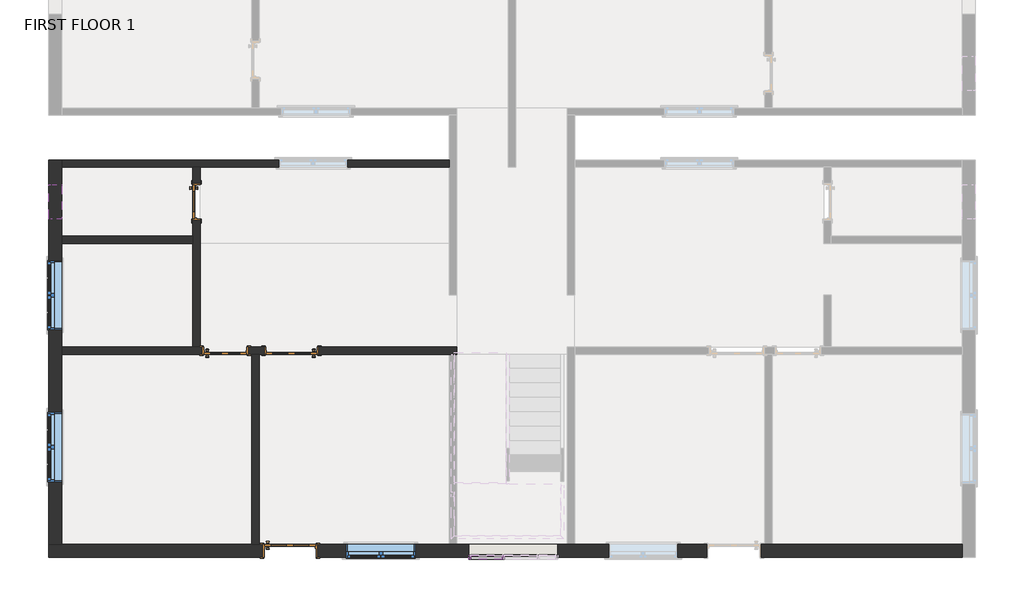
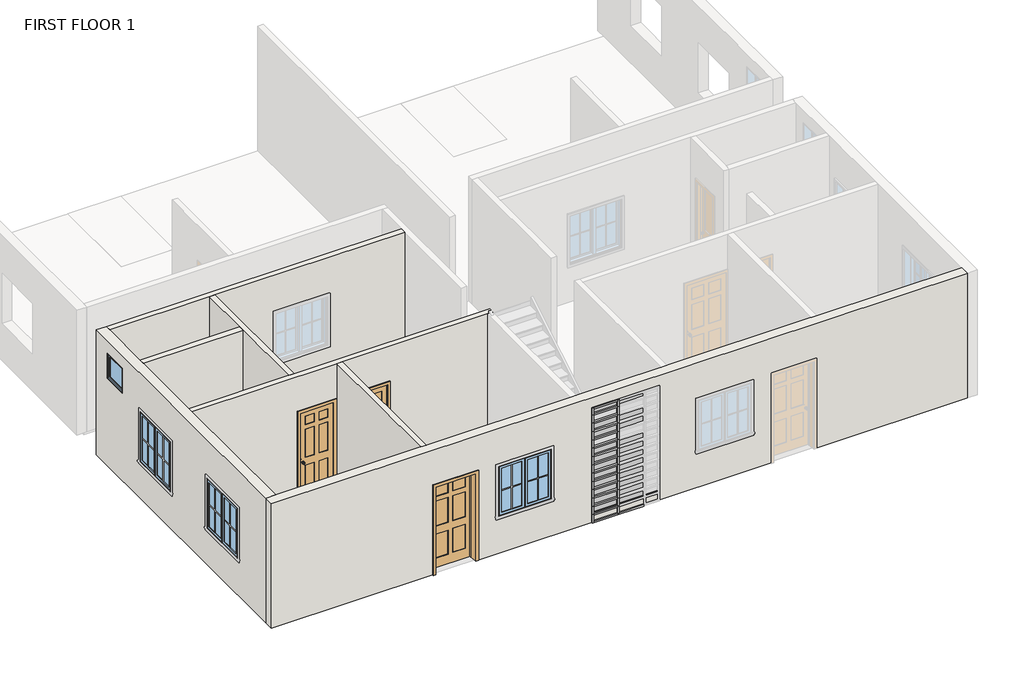
# One storey, part 1 of 4: 44 members, 24 plates, 7 walls, 4 doors, 4 windows.
"""IFC4 building model written with IfcOpenShell, lengths in millimetres."""

from ifc_helpers import new_model, si_unit, frame, origin, place, context, project, spatial, polyline, outline, extrude, faceted_brep, transform, mapped, element, save
from components import door_e337afa5, door_3b50870b, door_d86b6c54, door_03e3dfb5, member_56b223d9, member_a59c64b1, member_fa69921b, member_a67f877f, member_6a7c88b6, member_dc11c383, member_ff422208, system_panel_glazed_844a74e3, system_panel_glazed_a39216e9, system_panel_glazed_b3845325, system_panel_glazed_23b8b45c, system_panel_glazed_26c33eb0, system_panel_glazed_afc0885c, window_80340324, window_9200f5ac

model = new_model("IFC4")

# Units and contexts
model_context = context("Model", 3, world=origin())
ifc_project = project(units=[si_unit("LENGTHUNIT", "METRE", prefix="MILLI")], contexts=[model_context])

# Site, building, storey
site = spatial("IfcSite", under=ifc_project)
building = spatial("IfcBuilding", under=site)
storey = spatial("IfcBuildingStorey", under=building, Name="FIRST FLOOR 1", Elevation=3200.4)

# Doors
placement = place(None, origin())
door_shape = door_e337afa5(model_context)
element("IfcDoor", 1, ObjectType="Door-Interior-Single-2_Panel-Wood : 24\" x 84\"", at=placement, inside=storey, context=model_context, shape_type="MappedRepresentation", body=[
    mapped(door_shape, transform((-9830.0887331, -1548.6593836, 3200.4), x_axis=(0.0, -1.0, 0.0), y_axis=(1.0, 0.0, 0.0), z_axis=(0.0, 0.0, 1.0))),
])
door_2_shape = door_3b50870b(model_context)
element("IfcDoor", 2, ObjectType="Door-Interior-Single-6_Panel-Wood : 30\" x 84\"", at=placement, inside=storey, context=model_context, shape_type="MappedRepresentation", body=[
    mapped(door_2_shape, transform((-9318.9137331, -4180.7343836, 3200.4), x_axis=(1.0, 0.0, 0.0), y_axis=(0.0, 1.0, 0.0), z_axis=(0.0, 0.0, 1.0))),
])
door_3_shape = door_d86b6c54(model_context)
element("IfcDoor", 3, ObjectType="Door-Interior-Single-6_Panel-Wood : 36\" x 84\"", at=placement, inside=storey, context=model_context, shape_type="MappedRepresentation", body=[
    mapped(door_3_shape, transform((-8175.9137331, -7704.9843836, 3200.4), x_axis=(1.0, 0.0, 0.0), y_axis=(0.0, 1.0, 0.0), z_axis=(0.0, 0.0, 1.0))),
])
door_4_shape = door_03e3dfb5(model_context)
element("IfcDoor", 4, ObjectType="Door-Interior-Single-6_Panel-Wood : 36\" x 84\"", at=placement, inside=storey, context=model_context, shape_type="MappedRepresentation", body=[
    mapped(door_4_shape, transform((-8150.5137331, -4180.7343836, 3200.4), x_axis=(-1.0, 0.0, 0.0), y_axis=(0.0, -1.0, 0.0), z_axis=(0.0, 0.0, 1.0))),
])

# Members
member_shape = member_56b223d9(model_context)
element("IfcMember", 5, ObjectType="Rectangular Mullion : 1.5\" x 2.5\" rectangular", at=placement, inside=storey, context=model_context, shape_type="MappedRepresentation", body=[
    mapped(member_shape, transform((-4416.6334597, -7822.4593836, 3200.4), x_axis=(1.0, 0.0, 0.0), y_axis=(0.0, -1.0, 0.0), z_axis=(0.0, 0.0, -1.0))),
])
element("IfcMember", 6, ObjectType="Rectangular Mullion : 1.5\" x 2.5\" rectangular", at=placement, inside=storey, context=model_context, shape_type="MappedRepresentation", body=[
    mapped(member_shape, transform((-4416.6334597, -7822.4593836, 3403.6), x_axis=(1.0, 0.0, 0.0), y_axis=(0.0, -1.0, 0.0), z_axis=(0.0, 0.0, -1.0))),
])
element("IfcMember", 7, ObjectType="Rectangular Mullion : 1.5\" x 2.5\" rectangular", at=placement, inside=storey, context=model_context, shape_type="MappedRepresentation", body=[
    mapped(member_shape, transform((-4416.6334597, -7822.4593836, 3606.8), x_axis=(1.0, 0.0, 0.0), y_axis=(0.0, -1.0, 0.0), z_axis=(0.0, 0.0, -1.0))),
])
element("IfcMember", 8, ObjectType="Rectangular Mullion : 1.5\" x 2.5\" rectangular", at=placement, inside=storey, context=model_context, shape_type="MappedRepresentation", body=[
    mapped(member_shape, transform((-4416.6334597, -7822.4593836, 3810.0), x_axis=(1.0, 0.0, 0.0), y_axis=(0.0, -1.0, 0.0), z_axis=(0.0, 0.0, -1.0))),
])
element("IfcMember", 9, ObjectType="Rectangular Mullion : 1.5\" x 2.5\" rectangular", at=placement, inside=storey, context=model_context, shape_type="MappedRepresentation", body=[
    mapped(member_shape, transform((-4416.6334597, -7822.4593836, 4013.2), x_axis=(1.0, 0.0, 0.0), y_axis=(0.0, -1.0, 0.0), z_axis=(0.0, 0.0, -1.0))),
])
element("IfcMember", 10, ObjectType="Rectangular Mullion : 1.5\" x 2.5\" rectangular", at=placement, inside=storey, context=model_context, shape_type="MappedRepresentation", body=[
    mapped(member_shape, transform((-4416.6334597, -7822.4593836, 4216.4), x_axis=(1.0, 0.0, 0.0), y_axis=(0.0, -1.0, 0.0), z_axis=(0.0, 0.0, -1.0))),
])
element("IfcMember", 11, ObjectType="Rectangular Mullion : 1.5\" x 2.5\" rectangular", at=placement, inside=storey, context=model_context, shape_type="MappedRepresentation", body=[
    mapped(member_shape, transform((-4416.6334597, -7822.4593836, 4419.6), x_axis=(1.0, 0.0, 0.0), y_axis=(0.0, -1.0, 0.0), z_axis=(0.0, 0.0, -1.0))),
])
element("IfcMember", 12, ObjectType="Rectangular Mullion : 1.5\" x 2.5\" rectangular", at=placement, inside=storey, context=model_context, shape_type="MappedRepresentation", body=[
    mapped(member_shape, transform((-4416.6334597, -7822.4593836, 4622.8), x_axis=(1.0, 0.0, 0.0), y_axis=(0.0, -1.0, 0.0), z_axis=(0.0, 0.0, -1.0))),
])
element("IfcMember", 13, ObjectType="Rectangular Mullion : 1.5\" x 2.5\" rectangular", at=placement, inside=storey, context=model_context, shape_type="MappedRepresentation", body=[
    mapped(member_shape, transform((-4416.6334597, -7822.4593836, 4826.0), x_axis=(1.0, 0.0, 0.0), y_axis=(0.0, -1.0, 0.0), z_axis=(0.0, 0.0, -1.0))),
])
element("IfcMember", 14, ObjectType="Rectangular Mullion : 1.5\" x 2.5\" rectangular", at=placement, inside=storey, context=model_context, shape_type="MappedRepresentation", body=[
    mapped(member_shape, transform((-4416.6334597, -7822.4593836, 5029.2), x_axis=(1.0, 0.0, 0.0), y_axis=(0.0, -1.0, 0.0), z_axis=(0.0, 0.0, -1.0))),
])
element("IfcMember", 15, ObjectType="Rectangular Mullion : 1.5\" x 2.5\" rectangular", at=placement, inside=storey, context=model_context, shape_type="MappedRepresentation", body=[
    mapped(member_shape, transform((-4416.6334597, -7822.4593836, 5232.4), x_axis=(1.0, 0.0, 0.0), y_axis=(0.0, -1.0, 0.0), z_axis=(0.0, 0.0, -1.0))),
])
element("IfcMember", 16, ObjectType="Rectangular Mullion : 1.5\" x 2.5\" rectangular", at=placement, inside=storey, context=model_context, shape_type="MappedRepresentation", body=[
    mapped(member_shape, transform((-4416.6334597, -7822.4593836, 5435.6), x_axis=(1.0, 0.0, 0.0), y_axis=(0.0, -1.0, 0.0), z_axis=(0.0, 0.0, -1.0))),
])
element("IfcMember", 17, ObjectType="Rectangular Mullion : 1.5\" x 2.5\" rectangular", at=placement, inside=storey, context=model_context, shape_type="MappedRepresentation", body=[
    mapped(member_shape, transform((-4416.6334597, -7822.4593836, 5638.8), x_axis=(1.0, 0.0, 0.0), y_axis=(0.0, -1.0, 0.0), z_axis=(0.0, 0.0, -1.0))),
])
member_2_shape = member_a59c64b1(model_context)
element("IfcMember", 18, ObjectType="Rectangular Mullion : 1.5\" x 2.5\" rectangular", at=placement, inside=storey, context=model_context, shape_type="MappedRepresentation", body=[
    mapped(member_2_shape, transform((-4416.6334597, -7822.4593836, 5842.0), x_axis=(1.0, 0.0, 0.0), y_axis=(0.0, -1.0, 0.0), z_axis=(0.0, 0.0, -1.0))),
])
member_3_shape = member_fa69921b(model_context)
element("IfcMember", 19, ObjectType="Rectangular Mullion : 1.5\" x 2.5\" rectangular", at=placement, inside=storey, context=model_context, shape_type="MappedRepresentation", body=[
    mapped(member_3_shape, transform((-4435.6834597, -7822.4593836, 6007.7826151), x_axis=(0.0, 0.0, 1.0), y_axis=(0.0, -1.0, 0.0), z_axis=(1.0, 0.0, 0.0))),
])
element("IfcMember", 20, ObjectType="Rectangular Mullion : 1.5\" x 2.5\" rectangular", at=placement, inside=storey, context=model_context, shape_type="MappedRepresentation", body=[
    mapped(member_3_shape, transform((-4988.13346, -7822.4593836, 3200.4), x_axis=(0.0, 0.0, -1.0), y_axis=(0.0, -1.0, 0.0), z_axis=(-1.0, 0.0, 0.0))),
])
member_4_shape = member_a67f877f(model_context)
element("IfcMember", 21, ObjectType="Rectangular Mullion : 1.5\" x 2.5\" rectangular", at=placement, inside=storey, context=model_context, shape_type="MappedRepresentation", body=[
    mapped(member_4_shape, transform((-4397.5834597, -7822.4593836, 3200.4), x_axis=(0.0, 0.0, -1.0), y_axis=(0.0, -1.0, 0.0), z_axis=(-1.0, 0.0, 0.0))),
])
member_5_shape = member_6a7c88b6(model_context)
element("IfcMember", 22, ObjectType="Rectangular Mullion : 1.5\" x 2.5\" rectangular", at=placement, inside=storey, context=model_context, shape_type="MappedRepresentation", body=[
    mapped(member_5_shape, transform((-4435.6834597, -7822.4593836, 3403.6), x_axis=(0.0, 0.0, 1.0), y_axis=(0.0, -1.0, 0.0), z_axis=(1.0, 0.0, 0.0))),
])
element("IfcMember", 23, ObjectType="Rectangular Mullion : 1.5\" x 2.5\" rectangular", at=placement, inside=storey, context=model_context, shape_type="MappedRepresentation", body=[
    mapped(member_5_shape, transform((-4435.6834597, -7822.4593836, 3606.8), x_axis=(0.0, 0.0, 1.0), y_axis=(0.0, -1.0, 0.0), z_axis=(1.0, 0.0, 0.0))),
])
element("IfcMember", 24, ObjectType="Rectangular Mullion : 1.5\" x 2.5\" rectangular", at=placement, inside=storey, context=model_context, shape_type="MappedRepresentation", body=[
    mapped(member_5_shape, transform((-4435.6834597, -7822.4593836, 3810.0), x_axis=(0.0, 0.0, 1.0), y_axis=(0.0, -1.0, 0.0), z_axis=(1.0, 0.0, 0.0))),
])
element("IfcMember", 25, ObjectType="Rectangular Mullion : 1.5\" x 2.5\" rectangular", at=placement, inside=storey, context=model_context, shape_type="MappedRepresentation", body=[
    mapped(member_5_shape, transform((-4435.6834597, -7822.4593836, 4013.2), x_axis=(0.0, 0.0, 1.0), y_axis=(0.0, -1.0, 0.0), z_axis=(1.0, 0.0, 0.0))),
])
element("IfcMember", 26, ObjectType="Rectangular Mullion : 1.5\" x 2.5\" rectangular", at=placement, inside=storey, context=model_context, shape_type="MappedRepresentation", body=[
    mapped(member_5_shape, transform((-4435.6834597, -7822.4593836, 4216.4), x_axis=(0.0, 0.0, 1.0), y_axis=(0.0, -1.0, 0.0), z_axis=(1.0, 0.0, 0.0))),
])
element("IfcMember", 27, ObjectType="Rectangular Mullion : 1.5\" x 2.5\" rectangular", at=placement, inside=storey, context=model_context, shape_type="MappedRepresentation", body=[
    mapped(member_5_shape, transform((-4435.6834597, -7822.4593836, 4419.6), x_axis=(0.0, 0.0, 1.0), y_axis=(0.0, -1.0, 0.0), z_axis=(1.0, 0.0, 0.0))),
])
element("IfcMember", 28, ObjectType="Rectangular Mullion : 1.5\" x 2.5\" rectangular", at=placement, inside=storey, context=model_context, shape_type="MappedRepresentation", body=[
    mapped(member_5_shape, transform((-4435.6834597, -7822.4593836, 4622.8), x_axis=(0.0, 0.0, 1.0), y_axis=(0.0, -1.0, 0.0), z_axis=(1.0, 0.0, 0.0))),
])
element("IfcMember", 29, ObjectType="Rectangular Mullion : 1.5\" x 2.5\" rectangular", at=placement, inside=storey, context=model_context, shape_type="MappedRepresentation", body=[
    mapped(member_5_shape, transform((-4435.6834597, -7822.4593836, 4826.0), x_axis=(0.0, 0.0, 1.0), y_axis=(0.0, -1.0, 0.0), z_axis=(1.0, 0.0, 0.0))),
])
element("IfcMember", 30, ObjectType="Rectangular Mullion : 1.5\" x 2.5\" rectangular", at=placement, inside=storey, context=model_context, shape_type="MappedRepresentation", body=[
    mapped(member_5_shape, transform((-4435.6834597, -7822.4593836, 5029.2), x_axis=(0.0, 0.0, 1.0), y_axis=(0.0, -1.0, 0.0), z_axis=(1.0, 0.0, 0.0))),
])
element("IfcMember", 31, ObjectType="Rectangular Mullion : 1.5\" x 2.5\" rectangular", at=placement, inside=storey, context=model_context, shape_type="MappedRepresentation", body=[
    mapped(member_5_shape, transform((-4435.6834597, -7822.4593836, 5232.4), x_axis=(0.0, 0.0, 1.0), y_axis=(0.0, -1.0, 0.0), z_axis=(1.0, 0.0, 0.0))),
])
element("IfcMember", 32, ObjectType="Rectangular Mullion : 1.5\" x 2.5\" rectangular", at=placement, inside=storey, context=model_context, shape_type="MappedRepresentation", body=[
    mapped(member_5_shape, transform((-4435.6834597, -7822.4593836, 5435.6), x_axis=(0.0, 0.0, 1.0), y_axis=(0.0, -1.0, 0.0), z_axis=(1.0, 0.0, 0.0))),
])
element("IfcMember", 33, ObjectType="Rectangular Mullion : 1.5\" x 2.5\" rectangular", at=placement, inside=storey, context=model_context, shape_type="MappedRepresentation", body=[
    mapped(member_5_shape, transform((-4435.6834597, -7822.4593836, 5638.8), x_axis=(0.0, 0.0, 1.0), y_axis=(0.0, -1.0, 0.0), z_axis=(1.0, 0.0, 0.0))),
])
element("IfcMember", 34, ObjectType="Rectangular Mullion : 1.5\" x 2.5\" rectangular", at=placement, inside=storey, context=model_context, shape_type="MappedRepresentation", body=[
    mapped(member_5_shape, transform((-4435.6834597, -7822.4593836, 5842.0), x_axis=(0.0, 0.0, 1.0), y_axis=(0.0, -1.0, 0.0), z_axis=(1.0, 0.0, 0.0))),
])
member_6_shape = member_dc11c383(model_context)
element("IfcMember", 35, ObjectType="Rectangular Mullion : 1.5\" x 2.5\" rectangular", at=placement, inside=storey, context=model_context, shape_type="MappedRepresentation", body=[
    mapped(member_6_shape, transform((-5026.23346, -7822.4593836, 6007.7826151), x_axis=(-1.0, 0.0, 0.0), y_axis=(0.0, -1.0, 0.0), z_axis=(0.0, 0.0, 1.0))),
])
member_7_shape = member_ff422208(model_context)
element("IfcMember", 36, ObjectType="Rectangular Mullion : 1.5\" x 2.5\" rectangular", at=placement, inside=storey, context=model_context, shape_type="MappedRepresentation", body=[
    mapped(member_7_shape, transform((-5026.23346, -7822.4593836, 3403.6), x_axis=(-1.0, 0.0, 0.0), y_axis=(0.0, -1.0, 0.0), z_axis=(0.0, 0.0, 1.0))),
])
element("IfcMember", 37, ObjectType="Rectangular Mullion : 1.5\" x 2.5\" rectangular", at=placement, inside=storey, context=model_context, shape_type="MappedRepresentation", body=[
    mapped(member_7_shape, transform((-5026.23346, -7822.4593836, 3606.8), x_axis=(-1.0, 0.0, 0.0), y_axis=(0.0, -1.0, 0.0), z_axis=(0.0, 0.0, 1.0))),
])
element("IfcMember", 38, ObjectType="Rectangular Mullion : 1.5\" x 2.5\" rectangular", at=placement, inside=storey, context=model_context, shape_type="MappedRepresentation", body=[
    mapped(member_7_shape, transform((-5026.23346, -7822.4593836, 3810.0), x_axis=(-1.0, 0.0, 0.0), y_axis=(0.0, -1.0, 0.0), z_axis=(0.0, 0.0, 1.0))),
])
element("IfcMember", 39, ObjectType="Rectangular Mullion : 1.5\" x 2.5\" rectangular", at=placement, inside=storey, context=model_context, shape_type="MappedRepresentation", body=[
    mapped(member_7_shape, transform((-5026.23346, -7822.4593836, 4013.2), x_axis=(-1.0, 0.0, 0.0), y_axis=(0.0, -1.0, 0.0), z_axis=(0.0, 0.0, 1.0))),
])
element("IfcMember", 40, ObjectType="Rectangular Mullion : 1.5\" x 2.5\" rectangular", at=placement, inside=storey, context=model_context, shape_type="MappedRepresentation", body=[
    mapped(member_7_shape, transform((-5026.23346, -7822.4593836, 4216.4), x_axis=(-1.0, 0.0, 0.0), y_axis=(0.0, -1.0, 0.0), z_axis=(0.0, 0.0, 1.0))),
])
element("IfcMember", 41, ObjectType="Rectangular Mullion : 1.5\" x 2.5\" rectangular", at=placement, inside=storey, context=model_context, shape_type="MappedRepresentation", body=[
    mapped(member_7_shape, transform((-5026.23346, -7822.4593836, 4419.6), x_axis=(-1.0, 0.0, 0.0), y_axis=(0.0, -1.0, 0.0), z_axis=(0.0, 0.0, 1.0))),
])
element("IfcMember", 42, ObjectType="Rectangular Mullion : 1.5\" x 2.5\" rectangular", at=placement, inside=storey, context=model_context, shape_type="MappedRepresentation", body=[
    mapped(member_7_shape, transform((-5026.23346, -7822.4593836, 4622.8), x_axis=(-1.0, 0.0, 0.0), y_axis=(0.0, -1.0, 0.0), z_axis=(0.0, 0.0, 1.0))),
])
element("IfcMember", 43, ObjectType="Rectangular Mullion : 1.5\" x 2.5\" rectangular", at=placement, inside=storey, context=model_context, shape_type="MappedRepresentation", body=[
    mapped(member_7_shape, transform((-5026.23346, -7822.4593836, 4826.0), x_axis=(-1.0, 0.0, 0.0), y_axis=(0.0, -1.0, 0.0), z_axis=(0.0, 0.0, 1.0))),
])
element("IfcMember", 44, ObjectType="Rectangular Mullion : 1.5\" x 2.5\" rectangular", at=placement, inside=storey, context=model_context, shape_type="MappedRepresentation", body=[
    mapped(member_7_shape, transform((-5026.23346, -7822.4593836, 5029.2), x_axis=(-1.0, 0.0, 0.0), y_axis=(0.0, -1.0, 0.0), z_axis=(0.0, 0.0, 1.0))),
])
element("IfcMember", 45, ObjectType="Rectangular Mullion : 1.5\" x 2.5\" rectangular", at=placement, inside=storey, context=model_context, shape_type="MappedRepresentation", body=[
    mapped(member_7_shape, transform((-5026.23346, -7822.4593836, 5232.4), x_axis=(-1.0, 0.0, 0.0), y_axis=(0.0, -1.0, 0.0), z_axis=(0.0, 0.0, 1.0))),
])
element("IfcMember", 46, ObjectType="Rectangular Mullion : 1.5\" x 2.5\" rectangular", at=placement, inside=storey, context=model_context, shape_type="MappedRepresentation", body=[
    mapped(member_7_shape, transform((-5026.23346, -7822.4593836, 5435.6), x_axis=(-1.0, 0.0, 0.0), y_axis=(0.0, -1.0, 0.0), z_axis=(0.0, 0.0, 1.0))),
])
element("IfcMember", 47, ObjectType="Rectangular Mullion : 1.5\" x 2.5\" rectangular", at=placement, inside=storey, context=model_context, shape_type="MappedRepresentation", body=[
    mapped(member_7_shape, transform((-5026.23346, -7822.4593836, 5638.8), x_axis=(-1.0, 0.0, 0.0), y_axis=(0.0, -1.0, 0.0), z_axis=(0.0, 0.0, 1.0))),
])
element("IfcMember", 48, ObjectType="Rectangular Mullion : 1.5\" x 2.5\" rectangular", at=placement, inside=storey, context=model_context, shape_type="MappedRepresentation", body=[
    mapped(member_7_shape, transform((-5026.23346, -7822.4593836, 5842.0), x_axis=(-1.0, 0.0, 0.0), y_axis=(0.0, -1.0, 0.0), z_axis=(0.0, 0.0, 1.0))),
])

# Plates
system_panel_glazed_shape = system_panel_glazed_844a74e3(model_context)
element("IfcPlate", 49, ObjectType="System Panel : Glazed", at=placement, inside=storey, context=model_context, shape_type="MappedRepresentation", body=[
    mapped(system_panel_glazed_shape, transform((-4711.9084599, -7822.4593836, 3238.5), x_axis=(1.0, 0.0, 0.0), y_axis=(0.0, 1.0, 0.0), z_axis=(0.0, 0.0, 1.0))),
])
system_panel_glazed_2_shape = system_panel_glazed_a39216e9(model_context)
element("IfcPlate", 50, ObjectType="System Panel : Glazed", at=placement, inside=storey, context=model_context, shape_type="MappedRepresentation", body=[
    mapped(system_panel_glazed_2_shape, transform((-4111.8334597, -7822.4593836, 3238.5), x_axis=(1.0, 0.0, 0.0), y_axis=(0.0, 1.0, 0.0), z_axis=(0.0, 0.0, 1.0))),
])
system_panel_glazed_3_shape = system_panel_glazed_b3845325(model_context)
element("IfcPlate", 51, ObjectType="System Panel : Glazed", at=placement, inside=storey, context=model_context, shape_type="MappedRepresentation", body=[
    mapped(system_panel_glazed_3_shape, transform((-4711.9084599, -7822.4593836, 3422.65), x_axis=(1.0, 0.0, 0.0), y_axis=(0.0, 1.0, 0.0), z_axis=(0.0, 0.0, 1.0))),
])
element("IfcPlate", 52, ObjectType="System Panel : Glazed", at=placement, inside=storey, context=model_context, shape_type="MappedRepresentation", body=[
    mapped(system_panel_glazed_3_shape, transform((-4711.9084599, -7822.4593836, 3625.85), x_axis=(1.0, 0.0, 0.0), y_axis=(0.0, 1.0, 0.0), z_axis=(0.0, 0.0, 1.0))),
])
element("IfcPlate", 53, ObjectType="System Panel : Glazed", at=placement, inside=storey, context=model_context, shape_type="MappedRepresentation", body=[
    mapped(system_panel_glazed_3_shape, transform((-4711.9084599, -7822.4593836, 4032.25), x_axis=(1.0, 0.0, 0.0), y_axis=(0.0, 1.0, 0.0), z_axis=(0.0, 0.0, 1.0))),
])
element("IfcPlate", 54, ObjectType="System Panel : Glazed", at=placement, inside=storey, context=model_context, shape_type="MappedRepresentation", body=[
    mapped(system_panel_glazed_3_shape, transform((-4711.9084599, -7822.4593836, 4235.45), x_axis=(1.0, 0.0, 0.0), y_axis=(0.0, 1.0, 0.0), z_axis=(0.0, 0.0, 1.0))),
])
element("IfcPlate", 55, ObjectType="System Panel : Glazed", at=placement, inside=storey, context=model_context, shape_type="MappedRepresentation", body=[
    mapped(system_panel_glazed_3_shape, transform((-4711.9084599, -7822.4593836, 4641.85), x_axis=(1.0, 0.0, 0.0), y_axis=(0.0, 1.0, 0.0), z_axis=(0.0, 0.0, 1.0))),
])
element("IfcPlate", 56, ObjectType="System Panel : Glazed", at=placement, inside=storey, context=model_context, shape_type="MappedRepresentation", body=[
    mapped(system_panel_glazed_3_shape, transform((-4711.9084599, -7822.4593836, 4845.05), x_axis=(1.0, 0.0, 0.0), y_axis=(0.0, 1.0, 0.0), z_axis=(0.0, 0.0, 1.0))),
])
element("IfcPlate", 57, ObjectType="System Panel : Glazed", at=placement, inside=storey, context=model_context, shape_type="MappedRepresentation", body=[
    mapped(system_panel_glazed_3_shape, transform((-4711.9084599, -7822.4593836, 5251.45), x_axis=(1.0, 0.0, 0.0), y_axis=(0.0, 1.0, 0.0), z_axis=(0.0, 0.0, 1.0))),
])
element("IfcPlate", 58, ObjectType="System Panel : Glazed", at=placement, inside=storey, context=model_context, shape_type="MappedRepresentation", body=[
    mapped(system_panel_glazed_3_shape, transform((-4711.9084599, -7822.4593836, 5454.65), x_axis=(1.0, 0.0, 0.0), y_axis=(0.0, 1.0, 0.0), z_axis=(0.0, 0.0, 1.0))),
])
element("IfcPlate", 59, ObjectType="System Panel : Glazed", at=placement, inside=storey, context=model_context, shape_type="MappedRepresentation", body=[
    mapped(system_panel_glazed_3_shape, transform((-4711.9084599, -7822.4593836, 3829.05), x_axis=(1.0, 0.0, 0.0), y_axis=(0.0, 1.0, 0.0), z_axis=(0.0, 0.0, 1.0))),
])
element("IfcPlate", 60, ObjectType="System Panel : Glazed", at=placement, inside=storey, context=model_context, shape_type="MappedRepresentation", body=[
    mapped(system_panel_glazed_3_shape, transform((-4711.9084599, -7822.4593836, 4438.65), x_axis=(1.0, 0.0, 0.0), y_axis=(0.0, 1.0, 0.0), z_axis=(0.0, 0.0, 1.0))),
])
system_panel_glazed_4_shape = system_panel_glazed_23b8b45c(model_context)
element("IfcPlate", 61, ObjectType="System Panel : Glazed", at=placement, inside=storey, context=model_context, shape_type="MappedRepresentation", body=[
    mapped(system_panel_glazed_4_shape, transform((-4111.8334597, -7822.4593836, 3422.65), x_axis=(1.0, 0.0, 0.0), y_axis=(0.0, 1.0, 0.0), z_axis=(0.0, 0.0, 1.0))),
])
element("IfcPlate", 62, ObjectType="System Panel : Glazed", at=placement, inside=storey, context=model_context, shape_type="MappedRepresentation", body=[
    mapped(system_panel_glazed_4_shape, transform((-4111.8334597, -7822.4593836, 3625.85), x_axis=(1.0, 0.0, 0.0), y_axis=(0.0, 1.0, 0.0), z_axis=(0.0, 0.0, 1.0))),
])
element("IfcPlate", 63, ObjectType="System Panel : Glazed", at=placement, inside=storey, context=model_context, shape_type="MappedRepresentation", body=[
    mapped(system_panel_glazed_4_shape, transform((-4111.8334597, -7822.4593836, 4032.25), x_axis=(1.0, 0.0, 0.0), y_axis=(0.0, 1.0, 0.0), z_axis=(0.0, 0.0, 1.0))),
])
element("IfcPlate", 64, ObjectType="System Panel : Glazed", at=placement, inside=storey, context=model_context, shape_type="MappedRepresentation", body=[
    mapped(system_panel_glazed_4_shape, transform((-4111.8334597, -7822.4593836, 4235.45), x_axis=(1.0, 0.0, 0.0), y_axis=(0.0, 1.0, 0.0), z_axis=(0.0, 0.0, 1.0))),
])
element("IfcPlate", 65, ObjectType="System Panel : Glazed", at=placement, inside=storey, context=model_context, shape_type="MappedRepresentation", body=[
    mapped(system_panel_glazed_4_shape, transform((-4111.8334597, -7822.4593836, 4641.85), x_axis=(1.0, 0.0, 0.0), y_axis=(0.0, 1.0, 0.0), z_axis=(0.0, 0.0, 1.0))),
])
element("IfcPlate", 66, ObjectType="System Panel : Glazed", at=placement, inside=storey, context=model_context, shape_type="MappedRepresentation", body=[
    mapped(system_panel_glazed_4_shape, transform((-4111.8334597, -7822.4593836, 4845.05), x_axis=(1.0, 0.0, 0.0), y_axis=(0.0, 1.0, 0.0), z_axis=(0.0, 0.0, 1.0))),
])
element("IfcPlate", 67, ObjectType="System Panel : Glazed", at=placement, inside=storey, context=model_context, shape_type="MappedRepresentation", body=[
    mapped(system_panel_glazed_4_shape, transform((-4111.8334597, -7822.4593836, 5251.45), x_axis=(1.0, 0.0, 0.0), y_axis=(0.0, 1.0, 0.0), z_axis=(0.0, 0.0, 1.0))),
])
element("IfcPlate", 68, ObjectType="System Panel : Glazed", at=placement, inside=storey, context=model_context, shape_type="MappedRepresentation", body=[
    mapped(system_panel_glazed_4_shape, transform((-4111.8334597, -7822.4593836, 5454.65), x_axis=(1.0, 0.0, 0.0), y_axis=(0.0, 1.0, 0.0), z_axis=(0.0, 0.0, 1.0))),
])
element("IfcPlate", 69, ObjectType="System Panel : Glazed", at=placement, inside=storey, context=model_context, shape_type="MappedRepresentation", body=[
    mapped(system_panel_glazed_4_shape, transform((-4111.8334597, -7822.4593836, 3829.05), x_axis=(1.0, 0.0, 0.0), y_axis=(0.0, 1.0, 0.0), z_axis=(0.0, 0.0, 1.0))),
])
element("IfcPlate", 70, ObjectType="System Panel : Glazed", at=placement, inside=storey, context=model_context, shape_type="MappedRepresentation", body=[
    mapped(system_panel_glazed_4_shape, transform((-4111.8334597, -7822.4593836, 4438.65), x_axis=(1.0, 0.0, 0.0), y_axis=(0.0, 1.0, 0.0), z_axis=(0.0, 0.0, 1.0))),
])
system_panel_glazed_5_shape = system_panel_glazed_26c33eb0(model_context)
element("IfcPlate", 71, ObjectType="System Panel : Glazed", at=placement, inside=storey, context=model_context, shape_type="MappedRepresentation", body=[
    mapped(system_panel_glazed_5_shape, transform((-4711.9084599, -7822.4593836, 5861.05), x_axis=(1.0, 0.0, 0.0), y_axis=(0.0, 1.0, 0.0), z_axis=(0.0, 0.0, 1.0))),
])
system_panel_glazed_6_shape = system_panel_glazed_afc0885c(model_context)
element("IfcPlate", 72, ObjectType="System Panel : Glazed", at=placement, inside=storey, context=model_context, shape_type="MappedRepresentation", body=[
    mapped(system_panel_glazed_6_shape, transform((-4111.8334597, -7822.4593836, 5861.05), x_axis=(1.0, 0.0, 0.0), y_axis=(0.0, 1.0, 0.0), z_axis=(0.0, 0.0, 1.0))),
])

# Walls
element("IfcWall", 73, ObjectType="Inner Wall 5\"", at=placement, inside=storey, context=model_context, shape_type="Brep", body=[
    faceted_brep([(-12201.8137331, -939.0593836, 3200.4), (-9890.4137331, -939.0593836, 3200.4), (-9763.4137331, -939.0593836, 3200.4), (-5369.2137331, -939.0593836, 3200.4), (-5369.2137331, -939.0593836, 6248.4), (-9763.4137331, -939.0593836, 6248.4), (-9890.4137331, -939.0593836, 6248.4), (-12201.8137331, -939.0593836, 6248.4), (-7159.9137331, -939.0593836, 5334.0), (-7159.9137331, -939.0593836, 4114.8), (-8379.1137331, -939.0593836, 4114.8), (-8379.1137331, -939.0593836, 5334.0), (-12201.8137331, -812.0593836, 3200.4), (-12201.8137331, -812.0593836, 6248.4), (-5369.2137331, -812.0593836, 6248.4), (-5369.2137331, -812.0593836, 3200.4), (-7159.9137331, -812.0593836, 5334.0), (-8379.1137331, -812.0593836, 5334.0), (-8379.1137331, -812.0593836, 4114.8), (-7159.9137331, -812.0593836, 4114.8)], [[[0, 1, 2, 3, 4, 5, 6, 7], [8, 9, 10, 11]], [[12, 13, 14, 15], [16, 17, 18, 19]], [[3, 2, 1, 0, 12, 15]], [[7, 6, 5, 4, 14, 13]], [[0, 7, 13, 12]], [[4, 3, 15, 14]], [[9, 8, 16, 19]], [[10, 9, 19, 18]], [[11, 10, 18, 17]], [[8, 11, 17, 16]]]),
])
element("IfcWall", 74, ObjectType="Inner Wall 5\"", at=placement, inside=storey, context=model_context, shape_type="SweptSolid", body=[
    extrude(outline(polyline([(-8722.0137331, -4241.0593836), (-8722.0137331, -7593.8593836), (-8849.0137331, -7593.8593836), (-8849.0137331, -4241.0593836), (-8722.0137331, -4241.0593836)])), frame((0.0, 0.0, 3200.4), z_axis=(0.0, 0.0, 1.0), x_axis=(1.0, 0.0, 0.0)), (0.0, 0.0, 1.0), 3048.0),
])
element("IfcWall", 75, ObjectType="Inner Wall 5\"", at=placement, inside=storey, context=model_context, shape_type="Brep", body=[
    faceted_brep([(-12201.8137331, -4114.0593836, 6248.4), (-9890.4137331, -4114.0593836, 6248.4), (-9763.4137331, -4114.0593836, 6248.4), (-5242.2137331, -4114.0593836, 6248.4), (-5242.2137331, -4114.0593836, 3200.4), (-7667.9137331, -4114.0593836, 3200.4), (-7667.9137331, -4114.0593836, 5359.4), (-8633.1137331, -4114.0593836, 5359.4), (-8633.1137331, -4114.0593836, 3200.4), (-8912.5137331, -4114.0593836, 3200.4), (-8912.5137331, -4114.0593836, 5359.4), (-9725.3137331, -4114.0593836, 5359.4), (-9725.3137331, -4114.0593836, 3200.4), (-9763.4137331, -4114.0593836, 3200.4), (-9890.4137331, -4114.0593836, 3200.4), (-12201.8137331, -4114.0593836, 3200.4), (-5242.2137331, -4241.0593836, 6248.4), (-5369.2137331, -4241.0593836, 6248.4), (-8722.0137331, -4241.0593836, 6248.4), (-8849.0137331, -4241.0593836, 6248.4), (-12201.8137331, -4241.0593836, 6248.4), (-12201.8137331, -4241.0593836, 3200.4), (-9725.3137331, -4241.0593836, 3200.4), (-9725.3137331, -4241.0593836, 5359.4), (-8912.5137331, -4241.0593836, 5359.4), (-8912.5137331, -4241.0593836, 3200.4), (-8849.0137331, -4241.0593836, 3200.4), (-8722.0137331, -4241.0593836, 3200.4), (-8633.1137331, -4241.0593836, 3200.4), (-8633.1137331, -4241.0593836, 5359.4), (-7667.9137331, -4241.0593836, 5359.4), (-7667.9137331, -4241.0593836, 3200.4), (-5369.2137331, -4241.0593836, 3200.4), (-5242.2137331, -4241.0593836, 3200.4)], [[[0, 1, 2, 3, 4, 5, 6, 7, 8, 9, 10, 11, 12, 13, 14, 15]], [[16, 17, 18, 19, 20, 21, 22, 23, 24, 25, 26, 27, 28, 29, 30, 31, 32, 33]], [[21, 15, 14, 13, 12, 22]], [[4, 33, 32, 31, 5]], [[25, 9, 8, 28, 27, 26]], [[3, 2, 1, 0, 20, 19, 18, 17, 16]], [[0, 15, 21, 20]], [[4, 3, 16, 33]], [[10, 9, 25, 24]], [[11, 10, 24, 23]], [[12, 11, 23, 22]], [[7, 29, 28, 8]], [[29, 7, 6, 30]], [[30, 6, 5, 31]]]),
])
element("IfcWall", 76, ObjectType="Inner Wall 5\"", at=placement, inside=storey, context=model_context, shape_type="Brep", body=[
    faceted_brep([(-9763.4137331, -939.0593836, 6248.4), (-9763.4137331, -4114.0593836, 6248.4), (-9763.4137331, -4114.0593836, 3200.4), (-9763.4137331, -1878.8593836, 3200.4), (-9763.4137331, -1878.8593836, 5359.4), (-9763.4137331, -1218.4593836, 5359.4), (-9763.4137331, -1218.4593836, 3200.4), (-9763.4137331, -939.0593836, 3200.4), (-9890.4137331, -4114.0593836, 6248.4), (-9890.4137331, -2285.2593836, 6248.4), (-9890.4137331, -2158.2593836, 6248.4), (-9890.4137331, -939.0593836, 6248.4), (-9890.4137331, -939.0593836, 3200.4), (-9890.4137331, -1218.4593836, 3200.4), (-9890.4137331, -1218.4593836, 5359.4), (-9890.4137331, -1878.8593836, 5359.4), (-9890.4137331, -1878.8593836, 3200.4), (-9890.4137331, -2158.2593836, 3200.4), (-9890.4137331, -2285.2593836, 3200.4), (-9890.4137331, -4114.0593836, 3200.4)], [[[0, 1, 2, 3, 4, 5, 6, 7]], [[8, 9, 10, 11, 12, 13, 14, 15, 16, 17, 18, 19]], [[2, 19, 18, 17, 16, 3]], [[12, 7, 6, 13]], [[1, 0, 11, 10, 9, 8]], [[2, 1, 8, 19]], [[0, 7, 12, 11]], [[15, 4, 3, 16]], [[4, 15, 14, 5]], [[5, 14, 13, 6]]]),
])
element("IfcWall", 77, ObjectType="Inner Wall 5\"", at=placement, inside=storey, context=model_context, shape_type="SweptSolid", body=[
    extrude(outline(polyline([(-12201.8137331, -2158.2593836), (-9890.4137331, -2158.2593836), (-9890.4137331, -2285.2593836), (-12201.8137331, -2285.2593836), (-12201.8137331, -2158.2593836)])), frame((0.0, 0.0, 3200.4), z_axis=(0.0, 0.0, 1.0), x_axis=(1.0, 0.0, 0.0)), (0.0, 0.0, 1.0), 3048.0),
])
element("IfcWall", 78, ObjectType="outer wall 9\"", at=placement, inside=storey, context=model_context, shape_type="Brep", body=[
    faceted_brep([(3673.1862669, -7822.4593836, 6248.4), (-12430.4137331, -7822.4593836, 6248.4), (-12430.4137331, -7822.4593836, 3200.4), (-8658.5137331, -7822.4593836, 3200.4), (-8658.5137331, -7822.4593836, 5359.4), (-7693.3137331, -7822.4593836, 5359.4), (-7693.3137331, -7822.4593836, 3200.4), (-835.3137331, -7822.4593836, 3200.4), (-835.3137331, -7822.4593836, 5359.4), (129.8862669, -7822.4593836, 5359.4), (129.8862669, -7822.4593836, 3200.4), (3673.1862669, -7822.4593836, 3200.4), (-2562.5137331, -7822.4593836, 5334.0), (-1343.3137331, -7822.4593836, 5334.0), (-1343.3137331, -7822.4593836, 4114.8), (-2562.5137331, -7822.4593836, 4114.8), (-7185.3137331, -7822.4593836, 5334.0), (-5966.1137331, -7822.4593836, 5334.0), (-5966.1137331, -7822.4593836, 4114.8), (-7185.3137331, -7822.4593836, 4114.8), (-5026.23346, -7822.4593836, 6007.7826151), (-3461.6513929, -7822.4593836, 6007.7826151), (-3461.6513929, -7822.4593836, 3434.9143269), (-5026.23346, -7822.4593836, 3434.9143269), (-12430.4137331, -7593.8593836, 6248.4), (-12201.8137331, -7593.8593836, 6248.4), (-8849.0137331, -7593.8593836, 6248.4), (-8722.0137331, -7593.8593836, 6248.4), (-5369.2137331, -7593.8593836, 6248.4), (-5242.2137331, -7593.8593836, 6248.4), (-3286.4137331, -7593.8593836, 6248.4), (-3159.4137331, -7593.8593836, 6248.4), (193.3862669, -7593.8593836, 6248.4), (320.3862669, -7593.8593836, 6248.4), (3673.1862669, -7593.8593836, 6248.4), (3673.1862669, -7593.8593836, 3200.4), (320.3862669, -7593.8593836, 3200.4), (193.3862669, -7593.8593836, 3200.4), (129.8862669, -7593.8593836, 3200.4), (129.8862669, -7593.8593836, 5359.4), (-835.3137331, -7593.8593836, 5359.4), (-835.3137331, -7593.8593836, 3200.4), (-3159.4137331, -7593.8593836, 3200.4), (-3286.4137331, -7593.8593836, 3200.4), (-5242.2137331, -7593.8593836, 3200.4), (-5369.2137331, -7593.8593836, 3200.4), (-7693.3137331, -7593.8593836, 3200.4), (-7693.3137331, -7593.8593836, 5359.4), (-8658.5137331, -7593.8593836, 5359.4), (-8658.5137331, -7593.8593836, 3200.4), (-8722.0137331, -7593.8593836, 3200.4), (-8849.0137331, -7593.8593836, 3200.4), (-12201.8137331, -7593.8593836, 3200.4), (-12430.4137331, -7593.8593836, 3200.4), (-2562.5137331, -7593.8593836, 5334.0), (-2562.5137331, -7593.8593836, 4114.8), (-1343.3137331, -7593.8593836, 4114.8), (-1343.3137331, -7593.8593836, 5334.0), (-7185.3137331, -7593.8593836, 5334.0), (-7185.3137331, -7593.8593836, 4114.8), (-5966.1137331, -7593.8593836, 4114.8), (-5966.1137331, -7593.8593836, 5334.0), (-3461.6513929, -7593.8593836, 6007.7826151), (-5026.23346, -7593.8593836, 6007.7826151), (-5026.23346, -7593.8593836, 3434.9143269), (-3461.6513929, -7593.8593836, 3434.9143269)], [[[0, 1, 2, 3, 4, 5, 6, 7, 8, 9, 10, 11], [12, 13, 14, 15], [16, 17, 18, 19], [20, 21, 22, 23]], [[24, 25, 26, 27, 28, 29, 30, 31, 32, 33, 34, 35, 36, 37, 38, 39, 40, 41, 42, 43, 44, 45, 46, 47, 48, 49, 50, 51, 52, 53], [54, 55, 56, 57], [58, 59, 60, 61], [62, 63, 64, 65]], [[2, 53, 52, 51, 50, 49, 3]], [[35, 11, 10, 38, 37, 36]], [[6, 46, 45, 44, 43, 42, 41, 7]], [[1, 0, 34, 33, 32, 31, 30, 29, 28, 27, 26, 25, 24]], [[2, 1, 24, 53]], [[0, 11, 35, 34]], [[5, 47, 46, 6]], [[47, 5, 4, 48]], [[48, 4, 3, 49]], [[40, 8, 7, 41]], [[8, 40, 39, 9]], [[9, 39, 38, 10]], [[55, 54, 12, 15]], [[56, 55, 15, 14]], [[57, 56, 14, 13]], [[54, 57, 13, 12]], [[59, 58, 16, 19]], [[60, 59, 19, 18]], [[61, 60, 18, 17]], [[58, 61, 17, 16]], [[20, 63, 62, 21]], [[22, 65, 64, 23]], [[63, 20, 23, 64]], [[21, 62, 65, 22]]]),
])
element("IfcWall", 79, ObjectType="outer wall 9\"", at=placement, inside=storey, context=model_context, shape_type="Brep", body=[
    faceted_brep([(-12430.4137331, -812.0593836, 3200.4), (-12430.4137331, -7593.8593836, 3200.4), (-12430.4137331, -7593.8593836, 6248.4), (-12430.4137331, -812.0593836, 6248.4), (-12430.4137331, -5269.7593836, 5334.0), (-12430.4137331, -6488.9593836, 5334.0), (-12430.4137331, -6488.9593836, 4114.8), (-12430.4137331, -5269.7593836, 4114.8), (-12430.4137331, -2590.0593836, 5334.0), (-12430.4137331, -3809.2593836, 5334.0), (-12430.4137331, -3809.2593836, 4114.8), (-12430.4137331, -2590.0593836, 4114.8), (-12430.4137331, -1243.8593836, 5943.6), (-12430.4137331, -1853.4593836, 5943.6), (-12430.4137331, -1853.4593836, 5334.0), (-12430.4137331, -1243.8593836, 5334.0), (-12201.8137331, -812.0593836, 3200.4), (-12201.8137331, -812.0593836, 6248.4), (-12201.8137331, -939.0593836, 6248.4), (-12201.8137331, -2158.2593836, 6248.4), (-12201.8137331, -2285.2593836, 6248.4), (-12201.8137331, -4114.0593836, 6248.4), (-12201.8137331, -4241.0593836, 6248.4), (-12201.8137331, -7593.8593836, 6248.4), (-12201.8137331, -7593.8593836, 3200.4), (-12201.8137331, -4241.0593836, 3200.4), (-12201.8137331, -4114.0593836, 3200.4), (-12201.8137331, -2285.2593836, 3200.4), (-12201.8137331, -2158.2593836, 3200.4), (-12201.8137331, -939.0593836, 3200.4), (-12201.8137331, -5269.7593836, 5334.0), (-12201.8137331, -5269.7593836, 4114.8), (-12201.8137331, -6488.9593836, 4114.8), (-12201.8137331, -6488.9593836, 5334.0), (-12201.8137331, -2590.0593836, 5334.0), (-12201.8137331, -2590.0593836, 4114.8), (-12201.8137331, -3809.2593836, 4114.8), (-12201.8137331, -3809.2593836, 5334.0), (-12201.8137331, -1243.8593836, 5943.6), (-12201.8137331, -1243.8593836, 5334.0), (-12201.8137331, -1853.4593836, 5334.0), (-12201.8137331, -1853.4593836, 5943.6)], [[[0, 1, 2, 3], [4, 5, 6, 7], [8, 9, 10, 11], [12, 13, 14, 15]], [[16, 17, 18, 19, 20, 21, 22, 23, 24, 25, 26, 27, 28, 29], [30, 31, 32, 33], [34, 35, 36, 37], [38, 39, 40, 41]], [[1, 0, 16, 29, 28, 27, 26, 25, 24]], [[3, 2, 23, 22, 21, 20, 19, 18, 17]], [[2, 1, 24, 23]], [[0, 3, 17, 16]], [[31, 30, 4, 7]], [[32, 31, 7, 6]], [[33, 32, 6, 5]], [[30, 33, 5, 4]], [[35, 34, 8, 11]], [[36, 35, 11, 10]], [[37, 36, 10, 9]], [[34, 37, 9, 8]], [[39, 38, 12, 15]], [[40, 39, 15, 14]], [[41, 40, 14, 13]], [[38, 41, 13, 12]]]),
])

# Windows
window_shape = window_80340324(model_context)
element("IfcWindow", 80, ObjectType="Fixed : 24\" x 24\"", at=placement, inside=storey, context=model_context, shape_type="MappedRepresentation", body=[
    mapped(window_shape, transform((-12316.1137331, -1510.5593836, 4419.6), x_axis=(0.0, 1.0, 0.0), y_axis=(-1.0, 0.0, 0.0), z_axis=(0.0, 0.0, 1.0))),
])
window_2_shape = window_9200f5ac(model_context)
element("IfcWindow", 81, ObjectType="Window-Casement-Double : 48\" x 48\"", at=placement, inside=storey, context=model_context, shape_type="MappedRepresentation", body=[
    mapped(window_2_shape, transform((-6575.7137331, -7708.1593836, 3200.4), x_axis=(-1.0, 0.0, 0.0), y_axis=(0.0, -1.0, 0.0), z_axis=(0.0, 0.0, 1.0))),
])
element("IfcWindow", 82, ObjectType="Window-Casement-Double : 48\" x 48\"", at=placement, inside=storey, context=model_context, shape_type="MappedRepresentation", body=[
    mapped(window_2_shape, transform((-12316.1137331, -5879.3593836, 3200.4), x_axis=(0.0, 1.0, 0.0), y_axis=(-1.0, 0.0, 0.0), z_axis=(0.0, 0.0, 1.0))),
])
element("IfcWindow", 83, ObjectType="Window-Casement-Double : 48\" x 48\"", at=placement, inside=storey, context=model_context, shape_type="MappedRepresentation", body=[
    mapped(window_2_shape, transform((-12316.1137331, -3199.6593836, 3200.4), x_axis=(0.0, 1.0, 0.0), y_axis=(-1.0, 0.0, 0.0), z_axis=(0.0, 0.0, 1.0))),
])

save(model, "model.ifc")

# Revit data of these elements
# Type "Door-Interior-Single-2_Panel-Wood : 24\" x 84\""
#   Type Mark = "10"
#   Assembly Code = "C1020300"
#   Analytic Construction = "Wooden"
#   Top Rail = 0' - 4 11/16"
#   Thickness = 0' - 1 3/8"
#   Thermal Resistance (R) = 2.5876 (h·ft²·°F)/BTU
#   Swing Angle [instance default] = 90.00°
#   Stiles = 0' - 4 3/4"
#   Rough Width = 2' - 2"
#   Rough Height = 7' - 1"
#   Lock Rail = 0' - 7 1/2"
#   Height = 7' - 0"
#   Width = 2' - 0"
#   Heat Transfer Coefficient (U) = 0.3865 BTU/(h·ft²·°F)
#   Bottom Rail = 0' - 9 1/8"
#   Trim Material = Cherry
#   Panel Material = Cherry
#   Frame Material = Cherry
#   Door Handle Material = Aluminum
#   Visual Light Transmittance = 0
#   Solar Heat Gain Coefficient = 0
#   Wall Closure = (empty or 0)
#   Function = (empty or 0)
# Type "Door-Interior-Single-6_Panel-Wood : 30\" x 84\""
#   Type Mark = "9"
#   Assembly Code = "C1020300"
#   Analytic Construction = "Wooden"
#   Top Rail = 0' - 4 11/16"
#   Top Panel = 0' - 8"
#   Thickness = 0' - 1 3/8"
#   Thermal Resistance (R) = 2.5876 (h·ft²·°F)/BTU
#   Swing Angle [instance default] = 90.00°
#   Stiles = 0' - 4 3/4"
#   Rough Width = 2' - 8"
#   Rough Height = 7' - 1"
#   Mullion = 0' - 4 1/2"
#   Lock Rail = 0' - 7 1/2"
#   Intermediate Rail = 0' - 4 1/2"
#   Height = 7' - 0"
#   Width = 2' - 6"
#   Heat Transfer Coefficient (U) = 0.3865 BTU/(h·ft²·°F)
#   Bottom Rail = 0' - 9 1/8"
#   Trim Material = Cherry
#   Panel Material = Cherry
#   Frame Material = Cherry
#   Door Handle Material = Aluminum
#   Visual Light Transmittance = 0
#   Solar Heat Gain Coefficient = 0
#   Wall Closure = (empty or 0)
#   Function = (empty or 0)
# Type "Door-Interior-Single-6_Panel-Wood : 36\" x 84\""
#   Type Mark = "8"
#   Assembly Code = "C1020300"
#   Analytic Construction = "Wooden"
#   Top Rail = 0' - 4 11/16"
#   Top Panel = 0' - 11"
#   Thickness = 0' - 1 3/8"
#   Thermal Resistance (R) = 2.5876 (h·ft²·°F)/BTU
#   Swing Angle [instance default] = 90.00°
#   Stiles = 0' - 4 3/4"
#   Rough Width = 3' - 2"
#   Rough Height = 7' - 1"
#   Mullion = 0' - 4 1/2"
#   Lock Rail = 0' - 7 1/2"
#   Intermediate Rail = 0' - 4 1/2"
#   Height = 7' - 0"
#   Width = 3' - 0"
#   Heat Transfer Coefficient (U) = 0.3865 BTU/(h·ft²·°F)
#   Bottom Rail = 0' - 9 1/8"
#   Trim Material = Cherry
#   Panel Material = Cherry
#   Frame Material = Cherry
#   Door Handle Material = Aluminum
#   Visual Light Transmittance = 0
#   Solar Heat Gain Coefficient = 0
#   Wall Closure = (empty or 0)
#   Function = (empty or 0)
# Type "Rectangular Mullion : 1.5\" x 2.5\" rectangular"
#   built-in parameter 1007304 = 0.208333 (stored number, unit not read)
#   built-in parameter 1007301 = 0.0625 (stored number, unit not read)
#   built-in parameter 1007300 = 0.0625 (stored number, unit not read)
# Type "System Panel : Glazed"
#   Construction Type Id = "GSP4R"
#   Analytic Construction = "1/8 in Pilkington single glazing"
#   Visual Light Transmittance = 0.9
#   Solar Heat Gain Coefficient = 0.86
#   Heat Transfer Coefficient (U) = 1.18115 BTU/(h·ft²·°F)
#   Define Thermal Properties by = 1
# Type "Inner Wall 5\""
#   Assembly Code = "B2010"
#   Layers, outside or top first: 0' - 5" "wall paint" (function 1)
# Type "outer wall 9\""
#   Assembly Code = "B2010"
#   Layers, outside or top first: 0' - 9" "wall paint" (function 1)
# Type "Fixed : 24\" x 24\""
#   Type Mark = "3"
#   Construction Type Id = "GSP4R"
#   Assembly Code = "B2020100"
#   Analytic Construction = "1/8 in Pilkington single glazing"
#   Visual Light Transmittance = 0.9
#   Solar Heat Gain Coefficient = 0.78
#   Heat Transfer Coefficient (U) = 0.6496 BTU/(h·ft²·°F)
#   Height = 2' - 0"
#   Default Sill Height = 3' - 0"
#   Width = 2' - 0"
#   Window Inset = 0' - 0 3/4"
#   Define Thermal Properties by = 1
#   Define Thermal Properties by = 1
#   Glass Pane Material = Glass
#   Sash Material = Sash
#   Wall Closure = (empty or 0)
# Type "Window-Casement-Double : 48\" x 48\""
#   Type Mark = "18"
#   Fire Rating = "0.5h"
#   Assembly Code = "B2020100"
#   Analytic Construction = "Double glazing - domestic"
#   Frame Extension [instance default] = 0' - 0 1/4"
#   Window Inset [instance default] = 0' - 0"
#   Wall Thickness [instance default] = 0' - 6"
#   Interior Wall Closure [instance default] = 0' - 2 1/4"
#   Half Width = 2' - 0"
#   Visual Light Transmittance = 0.81
#   Thermal Resistance (R) = 1.8146 (h·ft²·°F)/BTU
#   Solar Heat Gain Coefficient = 0.76
#   Rough Width = 4' - 0 1/2"
#   Rough Height = 4' - 0 1/2"
#   Height = 4' - 0"
#   Heat Transfer Coefficient (U) = 0.5511 BTU/(h·ft²·°F)
#   Exterior Wall Closure [instance default] = 0' - 1 1/4"
#   Extension Jamb [instance default] = 0' - 2 1/4"
#   Default Sill Height = 3' - 0"
#   Width = 4' - 0"
#   Muntin Visibility = yes
#   Interior Trim Visibility [instance default] = yes
#   Exterior Trim Visibility [instance default] = yes
#   Extension Jamb Visibility [instance default] = yes
#   Interior Trim Material = Wood - Stained
#   Muntin Pattern = Muntin Pattern_2x2 : Muntin Pattern_2x2
#   Interior Trim = Trim-Window-Interior-Flat : Picture Frame
#   Interior Frame Material = Wood - Stained
#   Glass Panel Material = Glass
#   Exterior Trim Material = Clad - White
#   Exterior Trim = Trim-Window-Exterior-Flat : with Sill
#   Exterior Frame Material = Clad - White
#   Wall Closure = (empty or 0)
# Element 1 (IfcDoor, "Door-Interior-Single-2_Panel-Wood : 24\" x 84\"")
#   Swing Angle = 90.00°
#   Phase Created = New Construction
#   Materials on its faces: "Cherry", "Aluminum"
# Element 2 (IfcDoor, "Door-Interior-Single-6_Panel-Wood : 30\" x 84\"")
#   Swing Angle = 90.00°
#   Phase Created = New Construction
#   Materials on its faces: "Cherry", "Aluminum"
# Elements 3, 4 (IfcDoor, "Door-Interior-Single-6_Panel-Wood : 36\" x 84\"")
#   Swing Angle = 90.00°
#   Phase Created = New Construction
#   Materials on its faces: "Cherry", "Aluminum"
# Elements 5, 6, 7, 8, 9, 10, 11, 12, 13, 14, 15, 16, 17, 18, 19, 20, 21, 22, 23, 24, 25, 26, 27, 28, 29, 30, 31, 32, 33, 34, 35, 36, 37, 38, 39, 40, 41, 42, 43, 44, 45, 46, 47, 48 (IfcMember, "Rectangular Mullion : 1.5\" x 2.5\" rectangular")
#   Phase Created = New Construction
#   Materials on its faces: "Aluminum"
# Elements 49, 50, 51, 52, 53, 54, 55, 56, 57, 58, 59, 60, 61, 62, 63, 64, 65, 66, 67, 68, 69, 70, 71, 72 (IfcPlate, "System Panel : Glazed")
#   Phase Created = New Construction
#   Materials on its faces: "Glass"
# Element 73 (IfcWall, "Inner Wall 5\"")
#   Top Offset = 0' - 0"
#   Base Offset = 0' - 0"
#   Unconnected Height = 10' - 0"
#   wall height = 10' - 0"
#   Phase Created = New Construction
#   Base Constraint = FIRST FLOOR 1
#   Materials on its faces: "wall paint", "Clad - White"
# Elements 74, 75, 76, 77 (IfcWall, "Inner Wall 5\"")
#   Top Offset = 0' - 0"
#   Base Offset = 0' - 0"
#   Unconnected Height = 10' - 0"
#   wall height = 10' - 0"
#   Phase Created = New Construction
#   Base Constraint = FIRST FLOOR 1
#   Materials on its faces: "wall paint"
# Elements 78, 79 (IfcWall, "outer wall 9\"")
#   Top Offset = 0' - 0"
#   Base Offset = 0' - 0"
#   Unconnected Height = 10' - 0"
#   wall height = 10' - 0"
#   Phase Created = New Construction
#   Base Constraint = FIRST FLOOR 1
#   Materials on its faces: "wall paint", "Clad - White"
# Element 80 (IfcWindow, "Fixed : 24\" x 24\"")
#   Mark = "44"
#   Phase Created = New Construction
#   Materials on its faces: "Sash", "Glass"
# Element 81 (IfcWindow, "Window-Casement-Double : 48\" x 48\"")
#   Mark = "35"
#   Window Inset = 0' - 0"
#   Interior Wall Closure = 0' - 2 1/4"
#   Frame Extension = 0' - 0 1/4"
#   Exterior Wall Closure = 0' - 1 1/4"
#   Interior Trim Visibility = yes
#   Exterior Trim Visibility = yes
#   Phase Created = New Construction
#   Materials on its faces: "Wood - Stained", "Glass", "Clad - White"
# Element 82 (IfcWindow, "Window-Casement-Double : 48\" x 48\"")
#   Mark = "36"
#   Window Inset = 0' - 0"
#   Interior Wall Closure = 0' - 2 1/4"
#   Frame Extension = 0' - 0 1/4"
#   Exterior Wall Closure = 0' - 1 1/4"
#   Interior Trim Visibility = yes
#   Exterior Trim Visibility = yes
#   Phase Created = New Construction
#   Materials on its faces: "Wood - Stained", "Glass", "Clad - White"
# Element 83 (IfcWindow, "Window-Casement-Double : 48\" x 48\"")
#   Mark = "37"
#   Window Inset = 0' - 0"
#   Interior Wall Closure = 0' - 2 1/4"
#   Frame Extension = 0' - 0 1/4"
#   Exterior Wall Closure = 0' - 1 1/4"
#   Interior Trim Visibility = yes
#   Exterior Trim Visibility = yes
#   Phase Created = New Construction
#   Materials on its faces: "Wood - Stained", "Glass", "Clad - White"
# Materials
#   "Cherry": class "Wood", colour RGB 226 177 128, transparency 0, Description = "Prunus Serotina", Cost = 0
#   "Aluminum": class "Metal", colour RGB 247 247 247, transparency 0, Description = "Aluminum 6061", Cost = 0
#   "wall paint": class "Generic", colour RGB 120 120 120, transparency 0, Cost = 0
#   "Glass": class "Glass", colour RGB 0 128 192, transparency 0.75, Description = "Soda Lime Glass", Cost = 0
#   "Sash": class "Wood", colour RGB 224 178 126, transparency 0, Cost = 0
#   "Wood - Stained": class "Wood", colour RGB 224 178 126, transparency 0, Cost = 0
#   "Clad - White": class "Wood", colour RGB 242 242 238, transparency 0, Cost = 0
